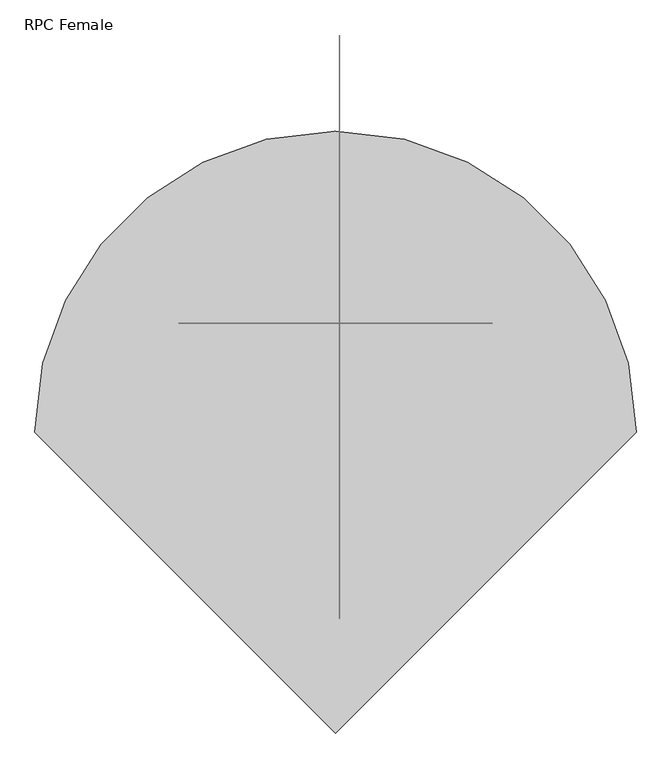
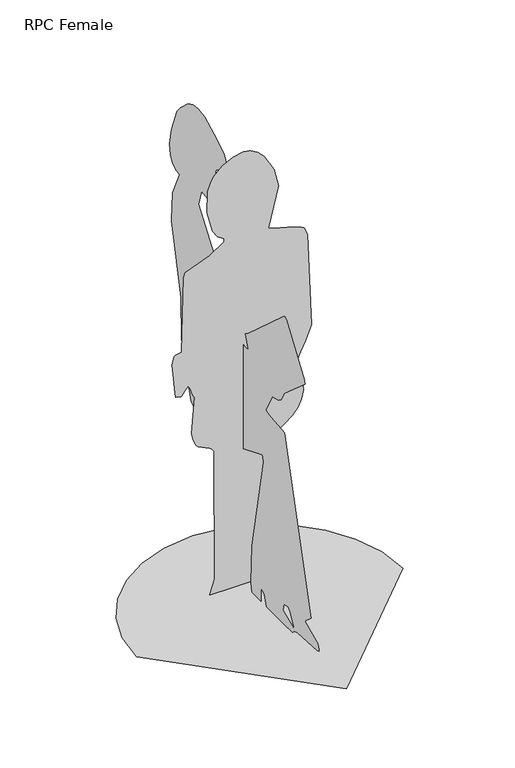
"""IFC4 building model written with IfcOpenShell, lengths in millimetres: proxy geometry, RPC Female."""

from ifc_helpers import new_model, si_unit, origin, place, context, project, spatial, triangles, source, transform, mapped, element, save


def rpc_female_69e001fa(model_context):
    return source(origin(), model_context, "Body", "Tessellation", [
        triangles([(441.0115623, 0.000195, 2.95e-05), (429.3526809, 101.0508723, 2.95e-05), (396.1482759, 193.849741, 2.95e-05), (344.0570151, 275.7380384, 2.95e-05), (275.7379839, 344.0571968, 2.95e-05), (193.8496139, 396.1483123, 2.95e-05), (101.0507542, 429.3527172, 2.95e-05), (0.0001128, 441.0116713, 2.95e-05), (-101.0505544, 429.3527899, 2.95e-05), (-193.8494322, 396.148385, 2.95e-05), (-275.7377296, 344.0571241, 2.95e-05), (-344.0569061, 275.7380929, 2.95e-05), (-396.1479853, 193.8497047, 2.95e-05), (-429.3523902, 101.050836, 2.95e-05), (-441.0113442, 0.0002072, 2.95e-05), (0.0001438, -441.0112716, 2.95e-05), (5.6288573, -72.8588658, 70.0852524), (5.6288585, -67.5989398, 46.4156806), (5.6288573, -125.4578945, 20.1161663), (5.6288573, -130.7178024, 25.3760469), (5.6288568, -108.5117995, 62.7542455), (5.6288568, -96.5284376, 75.3451376), (5.6288636, 28.8463111, 4.4e-06), (5.6288636, 40.229117, 35.8958717), (5.6288636, 42.8589028, 37.582617), (5.6288625, 46.0255291, 39.5148301), (5.628863, 49.4069043, 41.5083494), (5.628863, 52.681005, 43.379338), (5.628863, 55.5256987, 44.9433777), (5.628863, 57.6189803, 46.0169087), (5.628863, 58.6387491, 46.4156852), (5.6288642, 58.6388308, 5.3e-06), (5.628867, 109.8769052, 6.9e-06), (5.6288664, 117.5638814, 30.0747313), (5.6288619, 110.2503108, 165.0034458), (5.6288494, 45.8425779, 492.8873202), (5.6288488, 48.1189788, 514.5472627), (5.6288494, 53.3788639, 517.177153), (5.6288551, 178.1910311, 465.0429442), (5.6288659, 434.6626039, 445.1924844), (5.6288664, 450.5017533, 448.7984416), (5.6288659, 460.0242462, 459.6877842), (5.6288625, 516.0170857, 641.4428965), (5.628859, 518.8805374, 782.802364), (5.6288539, 571.5700902, 1021.0322994), (5.6288505, 566.21969, 1122.0662487), (5.628846, 526.7703175, 1208.8547012), (5.6288471, 549.382382, 1214.8042654), (5.6288471, 565.9655994, 1225.2772453), (5.6288471, 578.7778625, 1246.7330578), (5.628846, 582.3522446, 1283.6603096), (5.6288443, 571.2219646, 1340.5468082), (5.6288409, 539.9200962, 1421.8809425), (5.6288392, 521.1666261, 1445.9133419), (5.6288363, 476.5802487, 1486.8137524), (5.6288346, 449.7626269, 1499.3802818), (5.6288341, 419.2722642, 1503.8241966), (5.6288324, 384.616676, 1497.9941746), (5.6288307, 310.7213682, 1462.458989), (5.6288295, 273.9932867, 1438.4605991), (5.6288295, 262.185559, 1422.5043056), (5.6288307, 258.6746723, 1403.1431328), (5.6288318, 266.4050325, 1379.8015343), (5.6288318, 272.8454643, 1373.0538357), (5.6288341, 310.0952073, 1357.378775), (5.6288341, 316.3479143, 1352.4607613), (5.6288341, 319.0040749, 1345.6121967), (5.6288346, 317.1758071, 1332.7887062), (5.6288358, 305.8543688, 1300.9030071), (5.6288358, 306.5085803, 1292.1762142), (5.6288386, 347.7776456, 1237.8581635), (5.6288397, 353.1935214, 1227.2643333), (5.6288397, 357.0101126, 1223.4171844), (5.6288403, 363.9689901, 1222.1001137), (5.6288409, 400.532674, 1227.2643333), (5.6288431, 416.3123068, 1172.0353643), (5.6288437, 303.2702605, 1016.0021559), (5.6288454, 265.1504216, 911.3598513), (5.6288466, 263.775124, 856.4411104), (5.6288437, 152.5272633, 835.1195194), (5.6288426, 132.277491, 835.401479), (5.628842, 148.158462, 880.886566), (5.628842, 148.0571964, 882.7405226), (5.6288414, 137.6855366, 888.0610554), (5.6288284, -66.8523783, 1071.7676474), (5.6288278, -73.5721762, 1077.1684078), (5.6288273, -86.0403423, 1072.7861898), (5.6288284, -188.4956529, 924.5040344), (5.6288278, -191.2067156, 911.6700068), (5.6288358, -75.4888061, 809.1019215), (5.6288375, -53.9765018, 775.0415005), (5.628838, -41.2994232, 764.3927319), (5.6288397, -7.1097666, 756.5028791), (5.6288437, 31.0002698, 687.1164167), (5.6288437, 32.3392324, 682.8642054), (5.628842, 2.8209363, 678.8459913), (5.6288397, -75.4888061, 672.3443533), (5.6288505, -225.3960531, 114.7944466), (5.6288528, -193.9320943, 87.1596054), (5.6288528, -191.2067156, 83.2349994), (5.6288517, -259.585536, 54.3055515), (5.6288517, -263.2692319, 51.0626081), (5.6288511, -269.2554763, 42.3128878), (5.6288517, -272.6934387, 33.4609936), (5.6288517, -273.1919003, 30.0901578), (5.6288517, -272.7351876, 28.0059895), (5.6288522, -264.4336776, 24.8814686), (5.6288562, -149.6562449, 17.8736649), (5.6288573, -130.7178024, 12.2262931), (5.6288579, -120.2380551, 0.0), (104.0908666, 160.2089529, 3.1649078), (94.3579033, 160.2089529, 19.4060443), (89.3722792, 160.2089529, 24.6666948), (83.6749889, 160.2089529, 28.6502543), (77.3615298, 160.2089529, 30.6359184), (108.9209679, 160.208971, 488.2475235), (167.928994, 160.208971, 532.4711686), (185.1884419, 160.2089529, 554.3915603), (197.8182488, 160.2089529, 580.1067784), (203.7634891, 160.2089529, 609.7401077), (200.9693101, 160.2089529, 643.4147964), (182.2653646, 160.2089529, 694.762825), (181.0317008, 160.2089529, 706.1069727), (182.5596598, 160.2089529, 717.0533976), (187.6063721, 160.2089529, 730.9447008), (194.3765257, 160.2089529, 745.9818644), (210.3236083, 160.2089529, 778.2543858), (229.8987579, 160.2089529, 827.5114082), (217.4196868, 160.2089892, 1149.3768637), (206.2291816, 160.2089892, 1174.6651457), (197.3626625, 160.2089892, 1180.1408289), (179.9116746, 160.2089892, 1186.5602772), (157.4188797, 160.2090074, 1193.4647249), (133.4268122, 160.2090074, 1200.3943165), (111.4781428, 160.2090074, 1206.8904316), (95.1154424, 160.2090074, 1212.4937233), (87.8813364, 160.2090074, 1216.7444086), (122.0707194, 160.2090074, 1350.8719048), (106.8578307, 160.2090437, 1414.361198), (72.812575, 160.2090437, 1471.759584), (51.5733646, 160.2090437, 1493.1552258), (29.0406965, 160.2090437, 1507.0042351), (6.3528099, 160.2090437, 1511.2990311), (-28.6189517, 160.2090437, 1503.9375618), (-63.4776388, 160.2090437, 1485.8245686), (-92.9896819, 160.2090437, 1457.7803501), (-104.1052189, 160.2090437, 1440.290284), (-113.0716229, 160.2090437, 1412.8615803), (-115.1812325, 160.2090074, 1340.4901257), (-96.9761937, 160.2090074, 1269.5770123), (-80.5492803, 160.2090074, 1243.9710171), (-59.3960202, 160.2090074, 1229.89426), (-59.3960202, 160.2090074, 1219.3742626), (-106.3336349, 160.2090074, 1187.1321173), (-188.2636903, 160.2090255, 1156.2553682), (-192.5278195, 160.2090255, 1139.830426), (-199.1336482, 160.2090255, 881.9724009), (-218.9549129, 160.2090255, 877.9899405), (-221.2948136, 160.2090255, 876.8949492), (-223.230524, 160.2090255, 874.3329689), (-229.8985581, 160.2089892, 846.8826822), (-219.8231193, 160.2089892, 732.8331757), (-218.615544, 160.2089892, 731.6850626), (-200.1001226, 160.2089892, 727.4659161), (-198.783506, 160.2089892, 727.5732496), (-189.8889181, 160.2089892, 742.3224947), (-177.7438927, 160.2089892, 756.5027338), (-174.0054945, 160.2089892, 750.6861557), (-170.8934751, 160.208971, 743.8743622), (-168.1785245, 160.208971, 736.4751045), (-165.631369, 160.208971, 728.8964973), (-163.0227891, 160.208971, 721.5464373), (-160.1235293, 160.208971, 714.8328209), (-156.7042613, 160.208971, 709.1635448), (-165.9934653, 160.208971, 587.3215633), (-161.082228, 160.208971, 562.7220474), (-151.4443625, 160.208971, 540.8466748), (-144.6676413, 160.208971, 533.0879914), (-106.327031, 160.208971, 513.8626024), (-97.6973615, 160.208971, 507.5200027), (-90.955422, 160.208971, 498.7673756), (-89.4974987, 160.2089529, 49.829067), (-106.3299469, 160.2089529, 7.46e-05), (105.2757234, 160.2089529, 7.46e-05)], [[15, 16, 1], [14, 15, 1], [14, 1, 2], [13, 14, 2], [13, 2, 3], [13, 3, 4], [12, 13, 4], [11, 12, 4], [11, 4, 5], [11, 5, 6], [11, 6, 7], [11, 7, 8], [11, 8, 9], [11, 9, 10], [23, 17, 18], [110, 23, 18], [110, 18, 19], [109, 110, 19], [17, 23, 24], [31, 32, 33], [31, 33, 34], [109, 19, 20], [108, 109, 20], [88, 89, 90], [82, 83, 84], [85, 86, 87], [105, 106, 107], [104, 105, 107], [103, 104, 107], [102, 103, 107], [101, 102, 107], [100, 101, 107], [100, 107, 108], [100, 108, 20], [100, 20, 21], [100, 21, 22], [87, 88, 90], [85, 87, 90], [84, 85, 90], [84, 90, 91], [84, 91, 92], [84, 92, 93], [82, 84, 93], [81, 82, 93], [81, 93, 94], [80, 81, 94], [80, 94, 95], [99, 100, 22], [17, 24, 25], [17, 25, 26], [31, 34, 35], [30, 31, 35], [17, 26, 27], [17, 27, 28], [17, 28, 29], [29, 30, 35], [17, 29, 35], [22, 17, 35], [99, 22, 35], [98, 99, 35], [97, 98, 35], [97, 35, 36], [97, 36, 37], [96, 97, 37], [96, 37, 38], [95, 96, 38], [80, 95, 38], [80, 38, 39], [79, 80, 39], [79, 39, 40], [79, 40, 41], [79, 41, 42], [79, 42, 43], [79, 43, 44], [78, 79, 44], [77, 78, 44], [77, 44, 45], [77, 45, 46], [76, 77, 46], [76, 46, 47], [75, 76, 47], [72, 73, 74], [71, 72, 74], [61, 62, 63], [60, 61, 63], [60, 63, 64], [59, 60, 64], [59, 64, 65], [59, 65, 66], [58, 59, 66], [57, 58, 66], [56, 57, 66], [55, 56, 66], [54, 55, 66], [54, 66, 67], [53, 54, 67], [52, 53, 67], [52, 67, 68], [51, 52, 68], [50, 51, 68], [49, 50, 68], [48, 49, 68], [47, 48, 68], [75, 47, 68], [74, 75, 68], [71, 74, 68], [70, 71, 68], [69, 70, 68], [183, 184, 111], [183, 111, 112], [183, 112, 113], [183, 113, 114], [183, 114, 115], [182, 183, 115], [181, 182, 115], [181, 115, 116], [154, 155, 156], [164, 165, 166], [180, 181, 116], [163, 164, 166], [162, 163, 166], [162, 166, 167], [161, 162, 167], [160, 161, 167], [159, 160, 167], [158, 159, 167], [157, 158, 167], [180, 116, 117], [180, 117, 118], [180, 118, 119], [180, 119, 120], [180, 120, 121], [180, 121, 122], [179, 180, 122], [179, 122, 123], [178, 179, 123], [177, 178, 123], [176, 177, 123], [175, 176, 123], [174, 175, 123], [174, 123, 124], [174, 124, 125], [173, 174, 125], [172, 173, 125], [171, 172, 125], [170, 171, 125], [169, 170, 125], [169, 125, 126], [168, 169, 126], [168, 126, 127], [167, 168, 127], [157, 167, 127], [157, 127, 128], [156, 157, 128], [154, 156, 128], [153, 154, 128], [153, 128, 129], [153, 129, 130], [153, 130, 131], [153, 131, 132], [153, 132, 133], [153, 133, 134], [153, 134, 135], [153, 135, 136], [153, 136, 137], [152, 153, 137], [151, 152, 137], [150, 151, 137], [149, 150, 137], [149, 137, 138], [149, 138, 139], [148, 149, 139], [147, 148, 139], [146, 147, 139], [146, 139, 140], [145, 146, 140], [145, 140, 141], [144, 145, 141], [144, 141, 142], [144, 142, 143]], closed=False),
    ])


if __name__ == "__main__":
    model = new_model("IFC4")
    model_context = context("Model", 3, world=origin())
    ifc_project = project(units=[si_unit("LENGTHUNIT", "METRE", prefix="MILLI")], contexts=[model_context])
    site = spatial("IfcSite", under=ifc_project)
    building = spatial("IfcBuilding", under=site)
    placement = place(None, origin())
    rpc_female_shape = rpc_female_69e001fa(model_context)
    element("IfcBuildingElementProxy", 1, Name="RPC Female", ObjectType="RPC Female", at=placement, inside=building, context=model_context, shape_type="MappedRepresentation", body=[
        mapped(rpc_female_shape, transform((0.0, 0.0, 0.0), x_axis=(1.0, 0.0, 0.0), y_axis=(0.0, 1.0, 0.0), z_axis=(0.0, 0.0, 1.0))),
    ])
    save(model, "model.ifc")

# Revit data of these elements
# Type "RPC Female"
#   built-in parameter 1005195 = "RPC-8-FXA2-QQQ0-UGV2-6"
#   Height = 0
